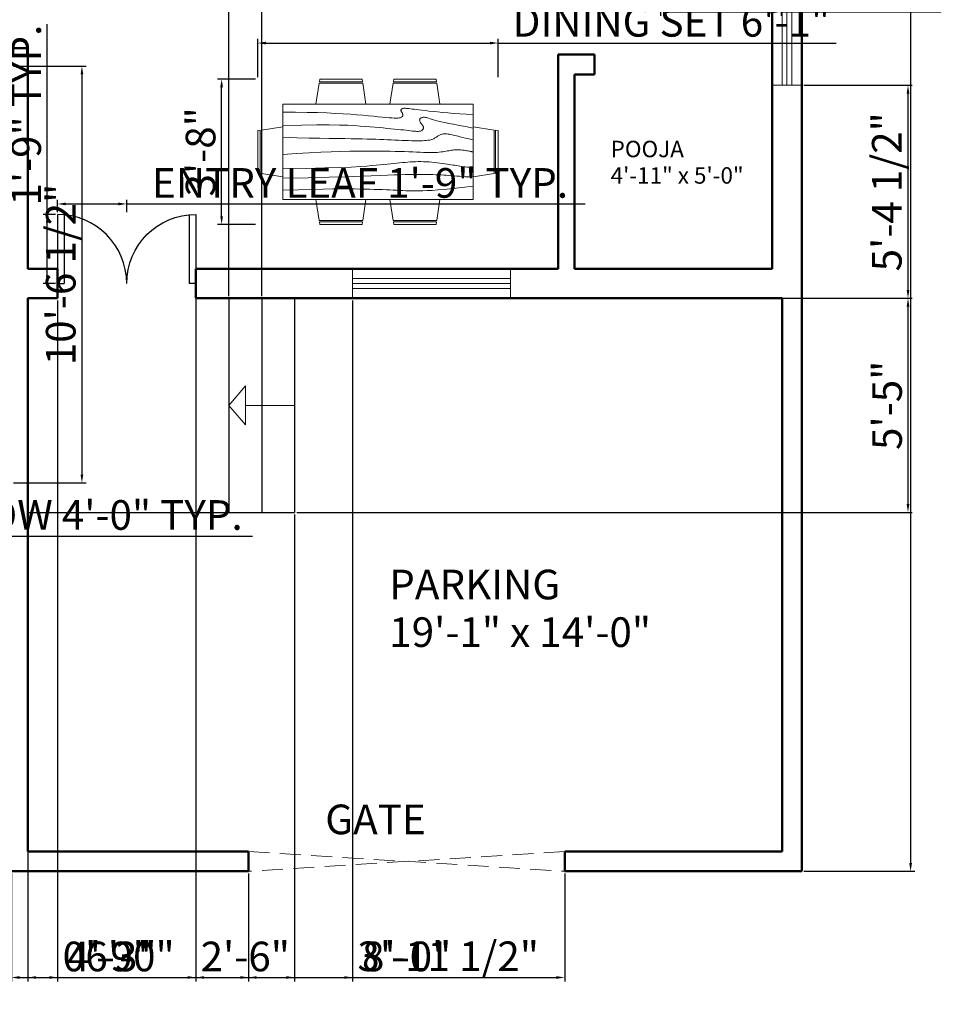
# Model space of a CAD drawing. Units: inches. Extents: x 2866 to 3545, y 873 to 1597.
# Tile 2 of 5: x 3186 to 3465, y 873 to 1172. Entities that reach past the tile are written whole.
import ezdxf

# ---------------------------------------------------------------- set-up
doc = ezdxf.new("R2010")
doc.units = ezdxf.units.IN
doc.linetypes.add('HIDDEN', pattern=[9.525, 6.35, -3.175])
doc.layers.add('A-ANNO-DIMS', color=152, linetype='Continuous', lineweight=18, true_color=0x2776bb)
for name, color, linetype, lineweight in [('A-ANNO-SYMB', 7, 'Continuous', 18), ('A-ANNO-TEXT', 7, 'Continuous', 25), ('A-AREA-IDEN', 7, 'Continuous', 25), ('A-DOOR', 3, 'Continuous', 25), ('A-DOOR-HIDN', 3, 'HIDDEN', 18), ('A-FLOR-STRS', 7, 'Continuous', 25), ('A-FURN', 8, 'Continuous', 18), ('A-GLAZ', 4, 'Continuous', 18), ('A-WALL', 7, 'Continuous', 50)]:
    doc.layers.add(name, color=color, linetype=linetype, lineweight=lineweight)
doc.styles.get("Standard").update_dxf_attribs({"font": 'arial.ttf'})
doc.dimstyles.new('ISO-25', dxfattribs={"dimtxt": 9, "dimasz": 2.5, "dimexe": 1.25, "dimexo": 0.625, "dimtad": 1, "dimdec": 0, "dimlunit": 3, "dimtxsty": 'Standard', "dimcen": 4.5, "dimadec": 0, "dimazin": 0, "dimtfac": 1, "dimtdec": 0, "dimtmove": 0, "dimatfit": 3, "dimfxl": 1, "dimarcsym": 0})

# ---------------------------------------------------------------- blocks, each defined once
blk = doc.blocks.new('Dining Set - 36 x 72 in.')
for p, q in [((-22, 27.5), (-22.1562, 26.50042)), ((-5.8416, 26.5), (-22.1534, 26.5)), ((-22, 27.5), (-6, 27.5)), ((-5.8437, 26.49966), (-6, 27.5)), ((6, 27.5), (5.8438, 26.50042)), ((22.1584, 26.5), (5.8466, 26.5)), ((6, 27.5), (22, 27.5)), ((22.1563, 26.49966), (22, 27.5)), ((-22.2343, 26.00059), (-23.4847, 17.99762)), ((-22.2304, 26), (-5.7608, 26)), ((-4.5152, 17.99762), (-5.7655, 25.99926)), ((5.7657, 26.00059), (4.5153, 17.99762)), ((5.7696, 26), (22.2392, 26)), ((23.4848, 17.99762), (22.2345, 25.99926)), ((36, 18), (-36, 18)), ((-36, 18), (-36, -18)), ((36, -18), (36, 18)), ((-45.5, 8), (-44.5004, 8.15617)), ((-45.5, 8), (-45.5, -8)), ((-44.5, -8.15843), (-44.5, 8.15338)), ((-44.0006, 8.23428), (-35.9976, 9.48474)), ((-44, 8.23041), (-44, -8.23915)), ((44.0006, 8.23428), (35.9976, 9.48474)), ((44, 8.23041), (44, -8.23915)), ((44.5, -8.15843), (44.5, 8.15338)), ((45.5, 8), (44.5005, 8.15617)), ((45.5, 8), (45.5, -8)), ((-44.4997, -8.15631), (-45.5, -8)), ((-35.9976, -9.48476), (-43.9993, -8.2345)), ((35.9976, -9.48476), (43.9993, -8.2345)), ((44.4997, -8.15631), (45.5, -8)), ((-36, -18), (36, -18)), ((-22.2343, -26.0006), (-23.4847, -17.99762)), ((-4.5152, -17.99762), (-5.7655, -25.99928)), ((5.7657, -26.0006), (4.5153, -17.99762)), ((23.4848, -17.99762), (22.2345, -25.99928)), ((-22.2304, -26), (-5.7608, -26)), ((5.7696, -26), (22.2392, -26)), ((-22, -27.5), (-22.1562, -26.50044)), ((-5.8416, -26.5), (-22.1534, -26.5)), ((-22, -27.5), (-6, -27.5)), ((-5.8437, -26.49967), (-6, -27.5)), ((6, -27.5), (5.8438, -26.50044)), ((22.1584, -26.5), (5.8466, -26.5)), ((6, -27.5), (22, -27.5)), ((22.1563, -26.49967), (22, -27.5))]:
    blk.add_line(p, q)
for points in [[(-36, 15), (-31.1772, 14.97754), (-26.8079, 14.91406), (-22.8538, 14.81543), (-19.276, 14.6875), (-16.0362, 14.53613), (-13.0957, 14.36718), (-10.4159, 14.18652), (-7.9583, 14), (-5.6904, 13.81315), (-3.6035, 13.63021), (-1.6954, 13.45508), (0.0365, 13.29166), (1.5945, 13.14388), (2.9811, 13.01562), (4.1988, 12.9108), (5.25, 12.83333), (6.1393, 12.78613), (6.8802, 12.76823), (7.4883, 12.77767), (7.9792, 12.8125), (8.3685, 12.87077), (8.6719, 12.95052), (8.9049, 13.0498), (9.0833, 13.16666), (9.2205, 13.29899), (9.3216, 13.44401), (9.3895, 13.59879), (9.4271, 13.76041), (9.4373, 13.92594), (9.4232, 14.09245), (9.3875, 14.257), (9.3333, 14.41666), (9.2638, 14.56917), (9.1836, 14.71484), (9.0975, 14.85465), (9.0104, 14.98958), (8.9272, 15.1206), (8.8529, 15.2487), (8.7922, 15.37483), (8.75, 15.5), (8.7305, 15.62467), (8.7344, 15.74739), (8.7617, 15.86621), (8.8125, 15.97916), (8.8867, 16.08431), (8.9844, 16.17968), (9.1055, 16.26334), (9.25, 16.33333), (9.4189, 16.38802), (9.6172, 16.42708), (9.8506, 16.45052), (10.125, 16.45833), (10.4463, 16.45052), (10.8203, 16.42708), (11.2529, 16.38802), (11.75, 16.33333), (12.3184, 16.26318), (12.9694, 16.17838), (13.7151, 16.07991), (14.5677, 15.96875), (15.5395, 15.84586), (16.6426, 15.71224), (17.8893, 15.56884), (19.2917, 15.41666), (20.859, 15.25667), (22.5879, 15.08984), (24.4721, 14.91715), (26.5052, 14.73958), (28.6809, 14.5581), (30.9929, 14.3737), (33.4347, 14.18733), (36, 14)], [(-36, 10), (-28.9766, 10.14274), (-23.1725, 10.20442), (-18.4241, 10.19775), (-14.5677, 10.13541), (-11.4399, 10.03011), (-8.877, 9.89453), (-6.7154, 9.74137), (-4.7917, 9.58333), (-2.9698, 9.43082), (-1.2246, 9.28515), (0.4415, 9.14534), (2.026, 9.01041), (3.5266, 8.87939), (4.9408, 8.7513), (6.266, 8.62516), (7.5, 8.5), (8.6411, 8.37549), (9.6914, 8.2539), (10.6538, 8.13818), (11.5312, 8.03125), (12.3267, 7.93603), (13.043, 7.85547), (13.6831, 7.79248), (14.25, 7.75), (14.7471, 7.7303), (15.1797, 7.73307), (15.5537, 7.75732), (15.875, 7.80208), (16.1494, 7.86637), (16.3828, 7.94922), (16.5811, 8.04964), (16.75, 8.16666), (16.8944, 8.29915), (17.0143, 8.44531), (17.1089, 8.60319), (17.1771, 8.77083), (17.218, 8.94629), (17.2305, 9.1276), (17.2137, 9.31282), (17.1667, 9.5), (17.0895, 9.6875), (16.987, 9.875), (16.8649, 10.0625), (16.7292, 10.25), (16.5856, 10.4375), (16.4401, 10.625), (16.2985, 10.8125), (16.1667, 11), (16.05, 11.18733), (15.9518, 11.3737), (15.8752, 11.5581), (15.8229, 11.73958), (15.798, 11.91715), (15.8034, 12.08984), (15.842, 12.25667), (15.9167, 12.41666), (16.0295, 12.56836), (16.1784, 12.70833), (16.3605, 12.83268), (16.5729, 12.9375), (16.8127, 13.01888), (17.0768, 13.07291), (17.3625, 13.0957), (17.6667, 13.08333), (17.9894, 13.03312), (18.3418, 12.94726), (18.7382, 12.82918), (19.1927, 12.68229), (19.7195, 12.51001), (20.3327, 12.31575), (21.0465, 12.10294), (21.875, 11.875), (22.8357, 11.63354), (23.959, 11.37304), (25.2786, 11.08618), (26.8282, 10.76562), (28.6414, 10.40405), (30.752, 9.99414), (33.1936, 9.52856), (36, 9)], [(-36, 5.5), (-30.7157, 5.3348), (-26.069, 5.20963), (-21.9946, 5.11767), (-18.4271, 5.05208), (-15.3009, 5.00602), (-12.5508, 4.97265), (-10.1112, 4.94515), (-7.9167, 4.91666), (-5.909, 4.88167), (-4.0586, 4.83984), (-2.3429, 4.79215), (-0.7396, 4.73958), (0.7739, 4.6831), (2.22, 4.6237), (3.6213, 4.56233), (5, 4.5), (6.373, 4.43782), (7.7344, 4.3776), (9.0723, 4.32129), (10.375, 4.27083), (11.6309, 4.22819), (12.8281, 4.19531), (13.9551, 4.17415), (15, 4.16666), (15.954, 4.17448), (16.819, 4.19791), (17.6001, 4.23698), (18.3021, 4.29166), (18.9299, 4.36198), (19.4883, 4.44791), (19.9823, 4.54948), (20.4167, 4.66666), (20.7969, 4.79899), (21.1302, 4.94401), (21.4245, 5.09879), (21.6875, 5.26041), (21.9271, 5.42594), (22.1511, 5.59245), (22.3672, 5.757), (22.5834, 5.91666), (22.8065, 6.06868), (23.0404, 6.21093), (23.2879, 6.34147), (23.5521, 6.45833), (23.8358, 6.55957), (24.142, 6.64323), (24.4735, 6.70735), (24.8334, 6.75), (25.2235, 6.76969), (25.642, 6.76692), (26.0858, 6.74267), (26.5521, 6.69791), (27.0379, 6.63362), (27.5404, 6.55078), (28.0565, 6.45036), (28.5834, 6.33333), (29.1242, 6.19987), (29.7071, 6.04687), (30.3661, 5.87044), (31.1354, 5.66666), (32.0493, 5.43164), (33.142, 5.16146), (34.4475, 4.85221), (36, 4.5)], [(-36, -1), (-30.7915, -0.6591), (-26.0195, -0.38216), (-21.6519, -0.16284), (-17.6563, 0.00521), (-14.0005, 0.12833), (-10.6523, 0.21289), (-7.5796, 0.26522), (-4.75, 0.29166), (-2.134, 0.29793), (0.2878, 0.28711), (2.5317, 0.26163), (4.6146, 0.22396), (6.5529, 0.17651), (8.3633, 0.12174), (10.0623, 0.06209), (11.6667, 0), (13.1899, -0.06201), (14.6341, -0.1211), (15.9982, -0.17432), (17.2813, -0.21875), (18.4823, -0.25147), (19.6003, -0.26953), (20.6343, -0.27002), (21.5834, -0.25), (22.4481, -0.20768), (23.2357, -0.14584), (23.9549, -0.06836), (24.6146, 0.02083), (25.2235, 0.11784), (25.7904, 0.21875), (26.3241, 0.31966), (26.8334, 0.41666), (27.3265, 0.50618), (27.8099, 0.58593), (28.2894, 0.65397), (28.7709, 0.70833), (29.2601, 0.74707), (29.763, 0.76823), (30.2855, 0.76985), (30.8334, 0.75), (31.4088, 0.70784), (31.9994, 0.64713), (32.589, 0.57275), (33.1615, 0.48958), (33.7008, 0.4025), (34.1908, 0.3164), (34.6153, 0.23616), (34.9584, 0.16666), (35.2099, 0.11165), (35.3848, 0.07031), (35.504, 0.04069), (35.5886, 0.02083), (35.6594, 0.00879), (35.7377, 0.0026), (35.8442, 0.00032), (36, 0)], [(-36, -6.5), (-27.1843, -6.31267), (-20.084, -6.1263), (-14.469, -5.9419), (-10.1094, -5.76042), (-6.7752, -5.58285), (-4.2363, -5.41016), (-2.2629, -5.24333), (-0.625, -5.08334), (0.8708, -4.93099), (2.2715, -4.78646), (3.5872, -4.64974), (4.8281, -4.52084), (6.0046, -4.39974), (7.127, -4.28646), (8.2053, -4.18099), (9.25, -4.08334), (10.2705, -3.99382), (11.2734, -3.91407), (12.2647, -3.84603), (13.25, -3.79167), (14.2354, -3.75293), (15.2266, -3.73177), (16.2295, -3.73015), (17.25, -3.75), (18.2912, -3.79248), (19.3451, -3.85547), (20.4009, -3.93604), (21.4479, -4.03125), (22.4754, -4.13819), (23.4727, -4.25391), (24.4289, -4.37549), (25.3334, -4.5), (26.1785, -4.62492), (26.9694, -4.74935), (27.7145, -4.87281), (28.4219, -4.99479), (29.1, -5.11483), (29.7572, -5.23242), (30.4016, -5.34709), (31.0417, -5.45834), (31.6837, -5.56437), (32.3262, -5.65821), (32.9658, -5.73153), (33.599, -5.77604), (34.2224, -5.78345), (34.8327, -5.74545), (35.4264, -5.65373), (36, -5.5)], [(-36, -10), (-26.4022, -9.81299), (-18.4675, -9.62891), (-11.9839, -9.45069), (-6.7396, -9.28125), (-2.5226, -9.12354), (0.8789, -8.98047), (3.6769, -8.85498), (6.0833, -8.75), (8.2767, -8.66765), (10.3021, -8.60677), (12.1712, -8.56543), (13.8958, -8.54167), (15.4876, -8.53353), (16.9583, -8.53907), (18.3197, -8.55632), (19.5834, -8.58334), (20.7616, -8.61841), (21.8685, -8.66081), (22.9188, -8.71004), (23.9271, -8.76563), (24.9081, -8.82707), (25.8763, -8.89388), (26.8465, -8.96558), (27.8334, -9.04167), (28.8474, -9.12118), (29.8828, -9.20117), (30.93, -9.27824), (31.9792, -9.34896), (33.0205, -9.40991), (34.0443, -9.45768), (35.0407, -9.48885), (36, -9.5)], [(-36, -14.5), (-30.0881, -14.33513), (-25.0332, -14.21224), (-20.7312, -14.12647), (-17.0781, -14.07292), (-13.97, -14.04671), (-11.3027, -14.04297), (-8.9724, -14.05681), (-6.875, -14.08334), (-4.9224, -14.11833), (-3.0905, -14.16016), (-1.3709, -14.20785), (0.2448, -14.26042), (1.7647, -14.3169), (3.1973, -14.3763), (4.5507, -14.43767), (5.8333, -14.5), (7.0554, -14.5621), (8.235, -14.62175), (9.3922, -14.67652), (10.5469, -14.72396), (11.7192, -14.76164), (12.929, -14.78711), (14.1965, -14.79794), (15.5417, -14.79167), (16.9933, -14.76424), (18.6152, -14.70508), (20.4804, -14.60197), (22.6615, -14.44271), (25.2312, -14.21509), (28.2624, -13.9069), (31.8277, -13.50594), (36, -13)]]:
    blk.add_lwpolyline(points)
blk = doc.blocks.new('*D19')
at = {"layer": 'A-ANNO-DIMS', "color": 0, "lineweight": -2, "transparency": 16777216}
for p, q in [((3423.67, 1523.69), (3457.33, 1523.69)), ((3456.08, 1521.19), (3456.08, 916.19)), ((3423.67, 913.69), (3457.33, 913.69))]:
    blk.add_line(p, q, dxfattribs=at)
at = {"layer": 'A-ANNO-DIMS', "color": 0, "transparency": 16777216}
for points in [[(3455.66, 1521.19), (3456.5, 1521.19), (3456.08, 1523.69)], [(3455.66, 916.19), (3456.5, 916.19), (3456.08, 913.69)]]:
    blk.add_solid(points, dxfattribs=at)
at = {"layer": 'Defpoints', "color": 0, "transparency": 16777216}
for p in [(3423.04, 1523.69), (3423.04, 913.69), (3456.08, 913.69)]:
    blk.add_point(p, dxfattribs=at)
at = {"layer": 'A-ANNO-DIMS', "color": 0, "transparency": 16777216, "insert": (3450.86, 1218.69), "char_height": 9, "attachment_point": 5, "rotation": 90}
blk.add_mtext('50\'-10"', dxfattribs=at)
blk = doc.blocks.new('WIN-48IN')
for p, q in [((0, 0), (0, 48)), ((0, 48), (9, 48)), ((3, 0), (3, 48)), ((4.5, 0), (4.5, 48)), ((6, 0), (6, 48)), ((9, 48), (9, 0)), ((9, 0), (0, 0))]:
    blk.add_line(p, q)
blk = doc.blocks.new('DOOR-ENTRY-LEAF-21IN')
for p, q in [((0, 21), (0, 0)), ((2, 21), (2, 0)), ((0, 0), (2, 0))]:
    blk.add_line(p, q)
blk.add_arc((0, 0), 21, 0, 90)
blk = doc.blocks.new('*D27')
at = {"layer": 'A-ANNO-DIMS', "color": 0, "lineweight": -2, "transparency": 16777216}
for p, q in [((3090.55, 1022.03), (3090.55, 1014.2)), ((3138.55, 1022.03), (3138.55, 1014.2)), ((3093.05, 1015.45), (3136.05, 1015.45)), ((3138.55, 1015.45), (3256.19, 1015.45))]:
    blk.add_line(p, q, dxfattribs=at)
at = {"layer": 'A-ANNO-DIMS', "color": 0, "transparency": 16777216}
for points in [[(3093.05, 1015.87), (3093.05, 1015.04), (3090.55, 1015.45)], [(3136.05, 1015.87), (3136.05, 1015.04), (3138.55, 1015.45)]]:
    blk.add_solid(points, dxfattribs=at)
at = {"layer": 'Defpoints', "color": 0, "transparency": 16777216}
for p in [(3090.55, 1022.65), (3138.55, 1022.65), (3138.55, 1015.45)]:
    blk.add_point(p, dxfattribs=at)
at = {"layer": 'A-ANNO-DIMS', "color": 0, "transparency": 16777216, "insert": (3198.62, 1020.73), "char_height": 9, "attachment_point": 5}
blk.add_mtext('WINDOW 4\'-0" TYP.', dxfattribs=at)
blk = doc.blocks.new('*D43')
at = {"layer": 'A-ANNO-DIMS', "color": 0, "lineweight": -2, "transparency": 16777216}
for p, q in [((3197.04, 1113.82), (3197.04, 1117.59)), ((3199.54, 1116.34), (3215.54, 1116.34)), ((3218.04, 1113.82), (3218.04, 1117.59)), ((3218.04, 1116.34), (3357.22, 1116.34))]:
    blk.add_line(p, q, dxfattribs=at)
at = {"layer": 'A-ANNO-DIMS', "color": 0, "transparency": 16777216}
for points in [[(3199.54, 1116.76), (3199.54, 1115.93), (3197.04, 1116.34)], [(3215.54, 1116.76), (3215.54, 1115.93), (3218.04, 1116.34)]]:
    blk.add_solid(points, dxfattribs=at)
at = {"layer": 'Defpoints', "color": 0, "transparency": 16777216}
for p in [(3218.04, 1116.34), (3197.04, 1113.19), (3218.04, 1113.19)]:
    blk.add_point(p, dxfattribs=at)
at = {"layer": 'A-ANNO-DIMS', "color": 0, "transparency": 16777216, "insert": (3288.88, 1121.56), "char_height": 9, "attachment_point": 5}
blk.add_mtext('ENTRY LEAF 1\'-9" TYP.', dxfattribs=at)
blk = doc.blocks.new('*D44')
at = {"layer": 'A-ANNO-DIMS', "color": 0, "lineweight": -2, "transparency": 16777216}
for p, q in [((3193.89, 1113.19), (3193.89, 1170.95)), ((3196.42, 1113.19), (3192.64, 1113.19)), ((3193.89, 1094.69), (3193.89, 1110.69)), ((3196.42, 1092.19), (3192.64, 1092.19))]:
    blk.add_line(p, q, dxfattribs=at)
at = {"layer": 'A-ANNO-DIMS', "color": 0, "transparency": 16777216}
for points in [[(3193.48, 1110.69), (3194.31, 1110.69), (3193.89, 1113.19)], [(3193.48, 1094.69), (3194.31, 1094.69), (3193.89, 1092.19)]]:
    blk.add_solid(points, dxfattribs=at)
at = {"layer": 'Defpoints', "color": 0, "transparency": 16777216}
for p in [(3193.89, 1113.19), (3197.04, 1113.19), (3197.04, 1092.19)]:
    blk.add_point(p, dxfattribs=at)
at = {"layer": 'A-ANNO-DIMS', "color": 0, "transparency": 16777216, "insert": (3188.67, 1143.32), "char_height": 9, "attachment_point": 5, "rotation": 90}
blk.add_mtext('1\'-9" TYP.', dxfattribs=at)
blk = doc.blocks.new('*D46')
at = {"layer": 'A-ANNO-DIMS', "color": 0, "lineweight": -2, "transparency": 16777216}
for p, q in [((3183.67, 1158.18), (3205.69, 1158.18)), ((3204.44, 1155.68), (3204.44, 1034.15)), ((3183.67, 1031.65), (3205.69, 1031.65))]:
    blk.add_line(p, q, dxfattribs=at)
at = {"layer": 'A-ANNO-DIMS', "color": 0, "transparency": 16777216}
for points in [[(3204.03, 1155.68), (3204.86, 1155.68), (3204.44, 1158.18)], [(3204.03, 1034.15), (3204.86, 1034.15), (3204.44, 1031.65)]]:
    blk.add_solid(points, dxfattribs=at)
at = {"layer": 'Defpoints', "color": 0, "transparency": 16777216}
for p in [(3183.04, 1158.18), (3183.04, 1031.65), (3204.44, 1031.65)]:
    blk.add_point(p, dxfattribs=at)
at = {"layer": 'A-ANNO-DIMS', "color": 0, "transparency": 16777216, "insert": (3199.17, 1094.92), "char_height": 9, "attachment_point": 5, "rotation": 90}
blk.add_mtext('10\'-6 1/2"', dxfattribs=at)
blk = doc.blocks.new('*D53')
at = {"layer": 'A-ANNO-DIMS', "color": 0, "lineweight": -2, "transparency": 16777216}
for p, q in [((3257.81, 1154.88), (3257.81, 1166.46)), ((3330.83, 1154.88), (3330.83, 1166.46)), ((3260.31, 1165.21), (3328.33, 1165.21)), ((3330.83, 1165.21), (3433.5, 1165.21))]:
    blk.add_line(p, q, dxfattribs=at)
at = {"layer": 'A-ANNO-DIMS', "color": 0, "transparency": 16777216}
for points in [[(3260.31, 1165.62), (3260.31, 1164.79), (3257.81, 1165.21)], [(3328.33, 1165.62), (3328.33, 1164.79), (3330.83, 1165.21)]]:
    blk.add_solid(points, dxfattribs=at)
at = {"layer": 'Defpoints', "color": 0, "transparency": 16777216}
for p in [(3330.83, 1165.21), (3257.81, 1154.25), (3330.83, 1154.25)]:
    blk.add_point(p, dxfattribs=at)
at = {"layer": 'A-ANNO-DIMS', "color": 0, "transparency": 16777216, "insert": (3383.42, 1170.48), "char_height": 9, "attachment_point": 5}
blk.add_mtext('DINING SET 6\'-1"', dxfattribs=at)
blk = doc.blocks.new('*D54')
at = {"layer": 'A-ANNO-DIMS', "color": 0, "lineweight": -2, "transparency": 16777216}
for p, q in [((3257.19, 1154.25), (3245.61, 1154.25)), ((3246.86, 1112.62), (3246.86, 1151.75)), ((3257.19, 1110.12), (3245.61, 1110.12))]:
    blk.add_line(p, q, dxfattribs=at)
at = {"layer": 'A-ANNO-DIMS', "color": 0, "transparency": 16777216}
for points in [[(3246.44, 1151.75), (3247.27, 1151.75), (3246.86, 1154.25)], [(3246.44, 1112.62), (3247.27, 1112.62), (3246.86, 1110.12)]]:
    blk.add_solid(points, dxfattribs=at)
at = {"layer": 'Defpoints', "color": 0, "transparency": 16777216}
for p in [(3246.86, 1154.25), (3257.81, 1154.25), (3257.81, 1110.12)]:
    blk.add_point(p, dxfattribs=at)
at = {"layer": 'A-ANNO-DIMS', "color": 0, "transparency": 16777216, "insert": (3241.63, 1132.18), "char_height": 9, "attachment_point": 5, "rotation": 90}
blk.add_mtext('3\'-8"', dxfattribs=at)
blk = doc.blocks.new('*D56')
at = {"layer": 'A-ANNO-DIMS', "color": 0, "lineweight": -2, "transparency": 16777216}
for p, q in [((3380.09, 1186.68), (3380.09, 1173.46)), ((3416.76, 1186.68), (3416.76, 1173.46)), ((3382.59, 1174.71), (3414.26, 1174.71)), ((3416.76, 1174.71), (3465.4, 1174.71))]:
    blk.add_line(p, q, dxfattribs=at)
at = {"layer": 'A-ANNO-DIMS', "color": 0, "transparency": 16777216}
for points in [[(3382.59, 1175.12), (3382.59, 1174.29), (3380.09, 1174.71)], [(3414.26, 1175.12), (3414.26, 1174.29), (3416.76, 1174.71)]]:
    blk.add_solid(points, dxfattribs=at)
at = {"layer": 'Defpoints', "color": 0, "transparency": 16777216}
for p in [(3380.09, 1187.31), (3416.76, 1187.31), (3416.76, 1174.71)]:
    blk.add_point(p, dxfattribs=at)
at = {"layer": 'A-ANNO-DIMS', "color": 0, "transparency": 16777216, "insert": (3442.33, 1179.99), "char_height": 9, "attachment_point": 5}
blk.add_mtext('3\'-0 1/2"', dxfattribs=at)
blk = doc.blocks.new('*D59')
at = {"layer": 'A-ANNO-DIMS', "color": 0, "lineweight": -2, "transparency": 16777216}
for p, q in [((3255.04, 913.07), (3255.04, 880.19)), ((3351.04, 913.07), (3351.04, 880.19)), ((3257.54, 881.44), (3348.54, 881.44))]:
    blk.add_line(p, q, dxfattribs=at)
at = {"layer": 'A-ANNO-DIMS', "color": 0, "transparency": 16777216}
for points in [[(3257.54, 881.86), (3257.54, 881.03), (3255.04, 881.44)], [(3348.54, 881.86), (3348.54, 881.03), (3351.04, 881.44)]]:
    blk.add_solid(points, dxfattribs=at)
at = {"layer": 'Defpoints', "color": 0, "transparency": 16777216}
for p in [(3255.04, 913.69), (3351.04, 913.69), (3351.04, 881.44)]:
    blk.add_point(p, dxfattribs=at)
at = {"layer": 'A-ANNO-DIMS', "color": 0, "transparency": 16777216, "insert": (3303.04, 886.66), "char_height": 9, "attachment_point": 5}
blk.add_mtext('8\'-0"', dxfattribs=at)
blk = doc.blocks.new('*D62')
at = {"layer": 'A-ANNO-DIMS', "color": 0, "lineweight": -2, "transparency": 16777216}
for p, q in [((3183.04, 913.07), (3183.04, 880.19)), ((3255.04, 913.07), (3255.04, 880.19)), ((3185.54, 881.44), (3252.54, 881.44))]:
    blk.add_line(p, q, dxfattribs=at)
at = {"layer": 'A-ANNO-DIMS', "color": 0, "transparency": 16777216}
for points in [[(3185.54, 881.86), (3185.54, 881.03), (3183.04, 881.44)], [(3252.54, 881.86), (3252.54, 881.03), (3255.04, 881.44)]]:
    blk.add_solid(points, dxfattribs=at)
at = {"layer": 'Defpoints', "color": 0, "transparency": 16777216}
for p in [(3183.04, 913.69), (3255.04, 913.69), (3255.04, 881.44)]:
    blk.add_point(p, dxfattribs=at)
at = {"layer": 'A-ANNO-DIMS', "color": 0, "transparency": 16777216, "insert": (3219.04, 886.66), "char_height": 9, "attachment_point": 5}
blk.add_mtext('6\'-0"', dxfattribs=at)
blk = doc.blocks.new('*D72')
at = {"layer": 'A-ANNO-DIMS', "color": 0, "lineweight": -2, "transparency": 16777216}
for p, q in [((3423.67, 1152.37), (3456.54, 1152.37)), ((3455.29, 1090.19), (3455.29, 1149.87)), ((3417.67, 1087.69), (3456.54, 1087.69))]:
    blk.add_line(p, q, dxfattribs=at)
at = {"layer": 'A-ANNO-DIMS', "color": 0, "transparency": 16777216}
for points in [[(3454.88, 1149.87), (3455.71, 1149.87), (3455.29, 1152.37)], [(3454.88, 1090.19), (3455.71, 1090.19), (3455.29, 1087.69)]]:
    blk.add_solid(points, dxfattribs=at)
at = {"layer": 'Defpoints', "color": 0, "transparency": 16777216}
for p in [(3423.04, 1152.37), (3455.29, 1152.37), (3417.04, 1087.69)]:
    blk.add_point(p, dxfattribs=at)
at = {"layer": 'A-ANNO-DIMS', "color": 0, "transparency": 16777216, "insert": (3450.01, 1120.03), "char_height": 9, "attachment_point": 5, "rotation": 90}
blk.add_mtext('5\'-4 1/2"', dxfattribs=at)
blk = doc.blocks.new('*D75')
at = {"layer": 'A-ANNO-DIMS', "color": 0, "lineweight": -2, "transparency": 16777216}
for p, q in [((3239.04, 1087.07), (3239.04, 880.19)), ((3286.6, 1087.07), (3286.6, 880.19)), ((3241.54, 881.44), (3284.1, 881.44)), ((3286.6, 881.44), (3342.23, 881.44))]:
    blk.add_line(p, q, dxfattribs=at)
at = {"layer": 'A-ANNO-DIMS', "color": 0, "transparency": 16777216}
for points in [[(3241.54, 881.86), (3241.54, 881.03), (3239.04, 881.44)], [(3284.1, 881.86), (3284.1, 881.03), (3286.6, 881.44)]]:
    blk.add_solid(points, dxfattribs=at)
at = {"layer": 'Defpoints', "color": 0, "transparency": 16777216}
for p in [(3239.04, 1087.69), (3286.6, 1087.69), (3286.6, 881.44)]:
    blk.add_point(p, dxfattribs=at)
at = {"layer": 'A-ANNO-DIMS', "color": 0, "transparency": 16777216, "insert": (3315.66, 886.72), "char_height": 9, "attachment_point": 5}
blk.add_mtext('3\'-11 1/2"', dxfattribs=at)
blk = doc.blocks.new('*D76')
at = {"layer": 'A-ANNO-DIMS', "color": 0, "lineweight": -2, "transparency": 16777216}
for p, q in [((3188.04, 1087.07), (3188.04, 880.19)), ((3197.04, 1087.07), (3197.04, 880.19)), ((3190.54, 881.44), (3194.54, 881.44)), ((3197.04, 881.44), (3224.72, 881.44))]:
    blk.add_line(p, q, dxfattribs=at)
at = {"layer": 'A-ANNO-DIMS', "color": 0, "transparency": 16777216}
for points in [[(3190.54, 881.86), (3190.54, 881.03), (3188.04, 881.44)], [(3194.54, 881.86), (3194.54, 881.03), (3197.04, 881.44)]]:
    blk.add_solid(points, dxfattribs=at)
at = {"layer": 'Defpoints', "color": 0, "transparency": 16777216}
for p in [(3188.04, 1087.69), (3197.04, 1087.69), (3197.04, 881.44)]:
    blk.add_point(p, dxfattribs=at)
at = {"layer": 'A-ANNO-DIMS', "color": 0, "transparency": 16777216, "insert": (3212.13, 886.66), "char_height": 9, "attachment_point": 5}
blk.add_mtext('0\'-9"', dxfattribs=at)
blk = doc.blocks.new('*D77')
at = {"layer": 'A-ANNO-DIMS', "color": 0, "lineweight": -2, "transparency": 16777216}
for p, q in [((3269.67, 1087.69), (3456.54, 1087.69)), ((3455.29, 1025.19), (3455.29, 1085.19)), ((3269.67, 1022.69), (3456.54, 1022.69))]:
    blk.add_line(p, q, dxfattribs=at)
at = {"layer": 'A-ANNO-DIMS', "color": 0, "transparency": 16777216}
for points in [[(3454.88, 1085.19), (3455.71, 1085.19), (3455.29, 1087.69)], [(3454.88, 1025.19), (3455.71, 1025.19), (3455.29, 1022.69)]]:
    blk.add_solid(points, dxfattribs=at)
at = {"layer": 'Defpoints', "color": 0, "transparency": 16777216}
for p in [(3269.04, 1087.69), (3455.29, 1087.69), (3269.04, 1022.69)]:
    blk.add_point(p, dxfattribs=at)
at = {"layer": 'A-ANNO-DIMS', "color": 0, "transparency": 16777216, "insert": (3450.09, 1055.19), "char_height": 9, "attachment_point": 5, "rotation": 90}
blk.add_mtext('5\'-5"', dxfattribs=at)
blk = doc.blocks.new('*D78')
at = {"layer": 'A-ANNO-DIMS', "color": 0, "lineweight": -2, "transparency": 16777216}
for p, q in [((3239.04, 1022.07), (3239.04, 880.19)), ((3269.04, 1022.07), (3269.04, 880.19)), ((3241.54, 881.44), (3266.54, 881.44))]:
    blk.add_line(p, q, dxfattribs=at)
at = {"layer": 'A-ANNO-DIMS', "color": 0, "transparency": 16777216}
for points in [[(3241.54, 881.86), (3241.54, 881.03), (3239.04, 881.44)], [(3266.54, 881.86), (3266.54, 881.03), (3269.04, 881.44)]]:
    blk.add_solid(points, dxfattribs=at)
at = {"layer": 'Defpoints', "color": 0, "transparency": 16777216}
for p in [(3239.04, 1022.69), (3269.04, 1022.69), (3269.04, 881.44)]:
    blk.add_point(p, dxfattribs=at)
at = {"layer": 'A-ANNO-DIMS', "color": 0, "transparency": 16777216, "insert": (3254.04, 886.66), "char_height": 9, "attachment_point": 5}
blk.add_mtext('2\'-6"', dxfattribs=at)
blk = doc.blocks.new('*D79')
at = {"layer": 'A-ANNO-DIMS', "color": 0, "lineweight": -2, "transparency": 16777216}
for p, q in [((3188.04, 1022.07), (3188.04, 880.19)), ((3239.04, 1022.07), (3239.04, 880.19)), ((3190.54, 881.44), (3236.54, 881.44))]:
    blk.add_line(p, q, dxfattribs=at)
at = {"layer": 'A-ANNO-DIMS', "color": 0, "transparency": 16777216}
for points in [[(3190.54, 881.86), (3190.54, 881.03), (3188.04, 881.44)], [(3236.54, 881.86), (3236.54, 881.03), (3239.04, 881.44)]]:
    blk.add_solid(points, dxfattribs=at)
at = {"layer": 'Defpoints', "color": 0, "transparency": 16777216}
for p in [(3188.04, 1022.69), (3239.04, 1022.69), (3239.04, 881.44)]:
    blk.add_point(p, dxfattribs=at)
at = {"layer": 'A-ANNO-DIMS', "color": 0, "transparency": 16777216, "insert": (3213.54, 886.66), "char_height": 9, "attachment_point": 5}
blk.add_mtext('4\'-3"', dxfattribs=at)
blk = doc.blocks.new('*D80')
at = {"layer": 'A-ANNO-DIMS', "color": 0, "lineweight": -2, "transparency": 16777216}
for p, q in [((3249.04, 1088.32), (3249.04, 1557.19)), ((3251.54, 1555.94), (3256.54, 1555.94)), ((3259.04, 1088.32), (3259.04, 1557.19)), ((3259.04, 1555.94), (3293.71, 1555.94))]:
    blk.add_line(p, q, dxfattribs=at)
at = {"layer": 'A-ANNO-DIMS', "color": 0, "transparency": 16777216}
for points in [[(3251.54, 1556.36), (3251.54, 1555.53), (3249.04, 1555.94)], [(3256.54, 1556.36), (3256.54, 1555.53), (3259.04, 1555.94)]]:
    blk.add_solid(points, dxfattribs=at)
at = {"layer": 'Defpoints', "color": 0, "transparency": 16777216}
for p in [(3259.04, 1555.94), (3249.04, 1087.69), (3259.04, 1087.69)]:
    blk.add_point(p, dxfattribs=at)
at = {"layer": 'A-ANNO-DIMS', "color": 0, "transparency": 16777216, "insert": (3277.63, 1561.16), "char_height": 9, "attachment_point": 5}
blk.add_mtext('0\'-10"', dxfattribs=at)

msp = doc.modelspace()

# ---------------------------------------------------------------- linework, layer by layer
at = {"layer": 'A-ANNO-SYMB'}
for p, q in [((3249.04, 1055.19), (3254.1, 1061.08)), ((3254.1, 1061.08), (3254.1, 1049.3)), ((3249.04, 1055.19), (3254.1, 1049.3)), ((3269.04, 1055.19), (3254.1, 1055.19))]:
    msp.add_line(p, q, dxfattribs=at)
at = {"layer": 'A-DOOR-HIDN'}
for p, q in [((3255.04, 919.69), (3351.04, 913.69)), ((3351.04, 919.69), (3255.04, 913.69))]:
    msp.add_line(p, q, dxfattribs=at)
at = {"layer": 'A-FLOR-STRS'}
for p, q in [((3239.04, 1087.69), (3239.04, 1022.69)), ((3249.04, 1087.69), (3249.04, 1022.69)), ((3259.04, 1087.69), (3259.04, 1022.69)), ((3269.04, 1087.69), (3269.04, 1022.69)), ((3188.04, 1022.69), (3239.04, 1022.69)), ((3239.04, 1022.69), (3269.04, 1022.69))]:
    msp.add_line(p, q, dxfattribs=at)
at = {"layer": 'A-WALL'}
for p, q in [((3423.04, 1523.69), (3423.04, 913.69)), ((3414.04, 1276.69), (3414.04, 1096.69)), ((3183.04, 1163.69), (3188.04, 1163.69)), ((3188.04, 1163.69), (3188.04, 1096.69)), ((3349.04, 1161.69), (3349.04, 1096.69)), ((3349.04, 1161.69), (3360.04, 1161.69)), ((3360.04, 1161.69), (3360.04, 1155.69)), ((3354.04, 1155.69), (3354.04, 1096.69)), ((3354.04, 1155.69), (3360.04, 1155.69)), ((3188.04, 1096.69), (3197.04, 1096.69)), ((3197.04, 1096.69), (3197.04, 1087.69)), ((3239.04, 1096.69), (3239.04, 1087.69)), ((3239.04, 1096.69), (3349.04, 1096.69)), ((3354.04, 1096.69), (3414.04, 1096.69)), ((3188.04, 1087.69), (3197.04, 1087.69)), ((3188.04, 1087.69), (3188.04, 919.69)), ((3239.04, 1087.69), (3417.04, 1087.69)), ((3417.04, 1087.69), (3417.04, 919.69)), ((3188.04, 919.69), (3255.04, 919.69)), ((3255.04, 913.69), (3255.04, 919.69)), ((3351.04, 913.69), (3351.04, 919.69)), ((3351.04, 919.69), (3417.04, 919.69)), ((3183.04, 913.69), (3255.04, 913.69)), ((3351.04, 913.69), (3423.04, 913.69))]:
    msp.add_line(p, q, dxfattribs=at)

# ---------------------------------------------------------------- block references
at = {"layer": 'A-DOOR'}
msp.add_blockref('DOOR-ENTRY-LEAF-21IN', (3197.04, 1092.19), dxfattribs=at)
at = {"layer": 'A-DOOR', "extrusion": (0, 0, -1), "zscale": -1}
msp.add_blockref('DOOR-ENTRY-LEAF-21IN', (-3239.04, 1092.19), dxfattribs=at)
at = {"layer": 'A-FURN', "xscale": 0.8024398644451542, "yscale": 0.8024398644451542, "zscale": 0.8024398644451542}
msp.add_blockref('Dining Set - 36 x 72 in.', (3294.32, 1132.18), dxfattribs=at)
at = {"layer": 'A-GLAZ'}
msp.add_blockref('WIN-48IN', (3414.04, 1152.37), dxfattribs=at)
at = {"layer": 'A-GLAZ', "rotation": 270}
msp.add_blockref('WIN-48IN', (3286.6, 1096.69), dxfattribs=at)

# ---------------------------------------------------------------- texts
at = {"layer": 'A-ANNO-TEXT'}
msp.add_text('GATE', height=9, dxfattribs=at).set_placement((3278.33, 924.95))
at = {"layer": 'A-AREA-IDEN'}
for s, height, p in [('POOJA ', 5, (3364.99, 1130.53)), ('4\'-11" x 5\'-0"', 5, (3364.99, 1122.5)), ('PARKING', 9, (3297.76, 996.28)), ('19\'-1" x 14\'-0"', 9, (3297.76, 981.82))]:
    msp.add_text(s, height=height, dxfattribs=at).set_placement(p)

# ---------------------------------------------------------------- dimensions: what is measured, and where the dimension line sits
at = {"layer": 'A-ANNO-DIMS'}
for base, p1, p2, picture, middle in [((3259.04, 1555.94), (3249.04, 1087.69), (3259.04, 1087.69), '*D80', (3277.63, 1561.16)), ((3416.76, 1174.71), (3380.09, 1187.31), (3416.76, 1187.31), '*D56', (3442.33, 1179.99)), ((3197.04, 881.44), (3188.04, 1087.69), (3197.04, 1087.69), '*D76', (3212.13, 886.66)), ((3286.6, 881.44), (3239.04, 1087.69), (3286.6, 1087.69), '*D75', (3315.66, 886.72)), ((3239.04, 881.44), (3188.04, 1022.69), (3239.04, 1022.69), '*D79', (3213.54, 886.66)), ((3269.04, 881.44), (3239.04, 1022.69), (3269.04, 1022.69), '*D78', (3254.04, 886.66)), ((3255.04, 881.44), (3183.04, 913.69), (3255.04, 913.69), '*D62', (3219.04, 886.66)), ((3351.04, 881.44), (3255.04, 913.69), (3351.04, 913.69), '*D59', (3303.04, 886.66))]:
    dim = msp.add_linear_dim(base=base, p1=p1, p2=p2, dimstyle='ISO-25', override={"dimdec": 1, "dimlfac": 1, "dimrnd": 0, "dimzin": 1, "dimdsep": 46, "dimlunit": 4, "dimfrac": 2}, dxfattribs=at)
    dim.commit()
    dim.dimension.update_dxf_attribs({"geometry": picture, "text_midpoint": middle})
for base, p1, p2, angle, override, picture, middle in [((3456.08, 913.69), (3423.04, 1523.69), (3423.04, 913.69), 90, {"dimclrd": 0, "dimclre": 0, "dimclrt": 0}, '*D19', (3450.86, 1218.69)), ((3204.44, 1031.65), (3183.04, 1158.18), (3183.04, 1031.65), 270, {"dimdec": 1, "dimlfac": 1, "dimrnd": 0, "dimzin": 1, "dimdsep": 46, "dimlunit": 4, "dimfrac": 2}, '*D46', (3199.17, 1094.92)), ((3246.86, 1154.25), (3257.81, 1110.12), (3257.81, 1154.25), 90, {"dimdec": 1, "dimlfac": 1, "dimrnd": 0, "dimzin": 1, "dimdsep": 46, "dimlunit": 4, "dimfrac": 2}, '*D54', (3241.63, 1132.18)), ((3455.29, 1152.37), (3417.04, 1087.69), (3423.04, 1152.37), 90, {"dimdec": 1, "dimlfac": 1, "dimrnd": 0, "dimzin": 1, "dimdsep": 46, "dimlunit": 4, "dimfrac": 2}, '*D72', (3450.01, 1120.03)), ((3455.29, 1087.69), (3269.04, 1022.69), (3269.04, 1087.69), 90, {"dimdec": 1, "dimlfac": 1, "dimrnd": 0, "dimzin": 1, "dimdsep": 46, "dimlunit": 4, "dimfrac": 2}, '*D77', (3450.09, 1055.19))]:
    dim = msp.add_linear_dim(base=base, p1=p1, p2=p2, angle=angle, dimstyle='ISO-25', override=override, dxfattribs=at)
    dim.commit()
    dim.dimension.update_dxf_attribs({"geometry": picture, "text_midpoint": middle})
for base, p1, p2, text, picture, middle in [((3330.83, 1165.21), (3257.81, 1154.25), (3330.83, 1154.25), 'DINING SET <>', '*D53', (3383.42, 1170.48)), ((3218.04, 1116.34), (3197.04, 1113.19), (3218.04, 1113.19), 'ENTRY LEAF <> TYP.', '*D43', (3288.88, 1121.56)), ((3138.55, 1015.45), (3090.55, 1022.65), (3138.55, 1022.65), 'WINDOW <> TYP.', '*D27', (3198.62, 1020.73))]:
    dim = msp.add_linear_dim(base=base, p1=p1, p2=p2, text=text, dimstyle='ISO-25', override={"dimdec": 1, "dimlfac": 1, "dimrnd": 0, "dimzin": 1, "dimdsep": 46, "dimlunit": 4, "dimfrac": 2}, dxfattribs=at)
    dim.commit()
    dim.dimension.update_dxf_attribs({"geometry": picture, "text_midpoint": middle})
dim = msp.add_linear_dim(base=(3193.89, 1113.19), p1=(3197.04, 1092.19), p2=(3197.04, 1113.19), angle=90, text='<> TYP.', dimstyle='ISO-25', override={"dimdec": 1, "dimlfac": 1, "dimrnd": 0, "dimzin": 1, "dimdsep": 46, "dimlunit": 4, "dimfrac": 2}, dxfattribs=at)
dim.commit()
dim.dimension.update_dxf_attribs({"geometry": '*D44', "text_midpoint": (3188.67, 1143.32)})

doc.saveas('drawing.dxf')
